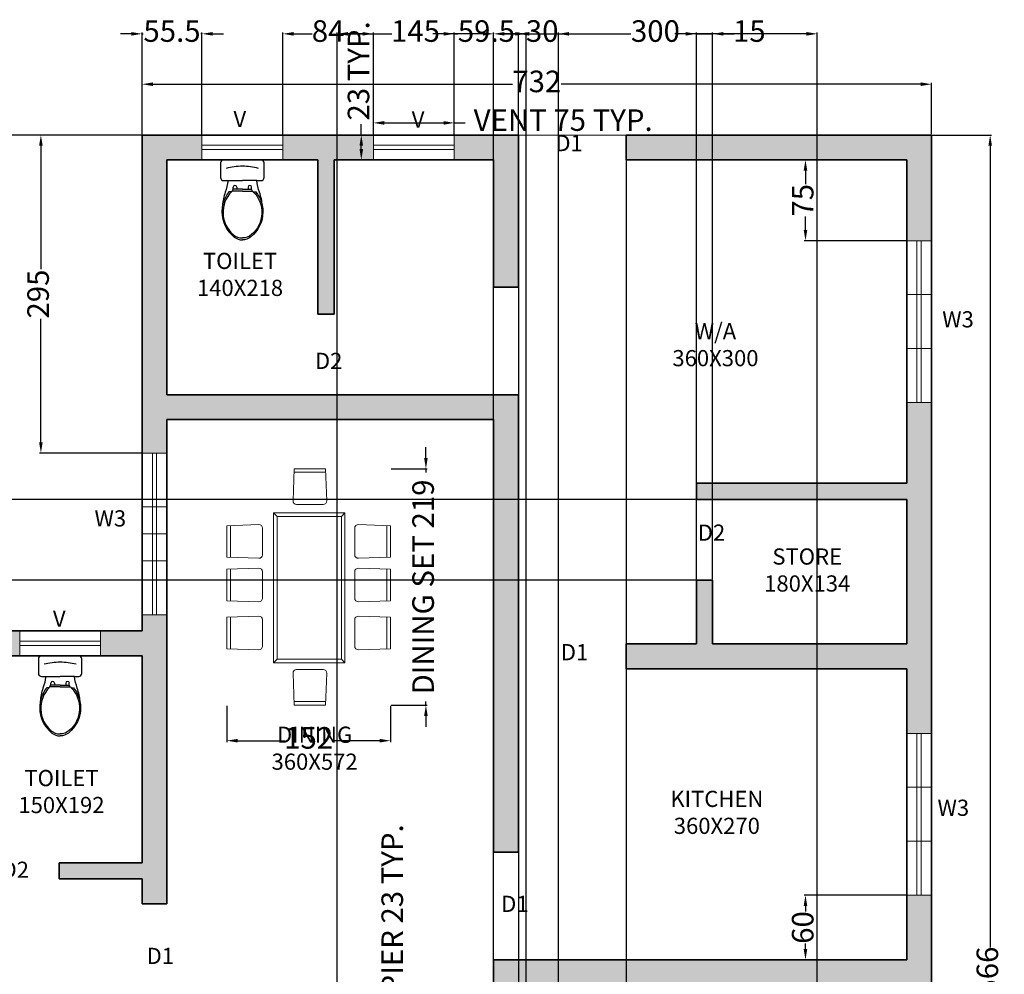
# Model space of a CAD drawing. Units: centimetres. Extents: x 2137 to 3697, y 183 to 2094.
# Tile 8 of 8: x 2745 to 3658, y 1208 to 2094. Entities that reach past the tile are written whole.
import ezdxf

# ---------------------------------------------------------------- set-up
doc = ezdxf.new("R2010")
doc.units = ezdxf.units.CM
for name, color, linetype, lineweight in [('A-ANNO-DIMS', 2, 'Continuous', 18), ('A-ANNO-TEXT', 7, 'Continuous', 18), ('A-AREA-IDEN', 7, 'Continuous', 25), ('A-DOOR', 3, 'Continuous', 18), ('A-FLOR-FIXT', 71, 'Continuous', 18), ('A-FURN', 8, 'Continuous', 18), ('A-GLAZ', 4, 'Continuous', 18), ('A-WALL', 7, 'Continuous', 35), ('A-WALL-PATT', 52, 'Continuous', 13)]:
    doc.layers.add(name, color=color, linetype=linetype, lineweight=lineweight)
doc.layers.add('WC-Detail_dwgmodels.com', color=251, linetype='Continuous')
doc.layers.add('WC-Outline_dwgmodels.com', color=250, linetype='Continuous')
doc.styles.get("Standard").update_dxf_attribs({"font": 'arial.ttf'})
doc.dimstyles.new('ISO-25', dxfattribs={"dimtxt": 20, "dimasz": 10, "dimexe": 1.25, "dimexo": 0.625, "dimtad": 0, "dimtxsty": 'Standard', "dimcen": 2.5, "dimadec": 0, "dimazin": 0, "dimtfac": 1, "dimtmove": 0, "dimatfit": 3, "dimfxl": 1, "dimarcsym": 0})

# ---------------------------------------------------------------- blocks, each defined once
blk = doc.blocks.new('*D1')
at = {"layer": 'A-ANNO-DIMS', "color": 0, "lineweight": -2, "transparency": 16777216}
for p, q in [((2858.02, 1987.3), (2858.02, 2034.96)), ((2868.02, 2033.71), (3201.49, 2033.71)), ((3580.02, 2033.71), (3246.56, 2033.71)), ((3590.02, 1987.3), (3590.02, 2034.96))]:
    blk.add_line(p, q, dxfattribs=at)
at = {"layer": 'A-ANNO-DIMS', "color": 0, "transparency": 16777216}
for points in [[(2868.02, 2035.37), (2868.02, 2032.04), (2858.02, 2033.71)], [(3580.02, 2035.37), (3580.02, 2032.04), (3590.02, 2033.71)]]:
    blk.add_solid(points, dxfattribs=at)
at = {"layer": 'Defpoints', "color": 0, "transparency": 16777216}
for p in [(3590.02, 2033.71), (2858.02, 1986.67), (3590.02, 1986.67)]:
    blk.add_point(p, dxfattribs=at)
at = {"layer": 'A-ANNO-DIMS', "color": 0, "transparency": 16777216, "insert": (3224.02, 2033.71), "char_height": 20, "attachment_point": 5}
blk.add_mtext('732', dxfattribs=at)
blk = doc.blocks.new('*D3')
at = {"layer": 'A-ANNO-DIMS', "color": 0, "lineweight": -2, "transparency": 16777216}
for p, q in [((3590.65, 1986.58), (3645.66, 1986.58)), ((3644.41, 1976.58), (3644.41, 1233.12)), ((3644.41, 430.58), (3644.41, 1174.04)), ((3590.65, 420.58), (3645.66, 420.58))]:
    blk.add_line(p, q, dxfattribs=at)
at = {"layer": 'A-ANNO-DIMS', "color": 0, "transparency": 16777216}
for points in [[(3642.74, 1976.58), (3646.07, 1976.58), (3644.41, 1986.58)], [(3642.74, 430.58), (3646.07, 430.58), (3644.41, 420.58)]]:
    blk.add_solid(points, dxfattribs=at)
at = {"layer": 'Defpoints', "color": 0, "transparency": 16777216}
for p in [(3590.02, 1986.58), (3644.41, 1986.58), (3590.02, 420.58)]:
    blk.add_point(p, dxfattribs=at)
at = {"layer": 'A-ANNO-DIMS', "color": 0, "transparency": 16777216, "insert": (3644.41, 1203.58), "char_height": 20, "attachment_point": 5, "rotation": 90}
blk.add_mtext('1566', dxfattribs=at)
blk = doc.blocks.new('*D6')
at = {"layer": 'A-ANNO-DIMS', "color": 0, "lineweight": -2, "transparency": 16777216}
for p, q in [((2857.4, 1986.58), (2218.37, 1986.58)), ((2219.62, 1976.58), (2219.62, 1779.67)), ((2219.62, 1536.58), (2219.62, 1733.49)), ((2857.4, 1526.58), (2218.37, 1526.58))]:
    blk.add_line(p, q, dxfattribs=at)
at = {"layer": 'A-ANNO-DIMS', "color": 0, "transparency": 16777216}
for points in [[(2217.95, 1976.58), (2221.28, 1976.58), (2219.62, 1986.58)], [(2217.95, 1536.58), (2221.28, 1536.58), (2219.62, 1526.58)]]:
    blk.add_solid(points, dxfattribs=at)
at = {"layer": 'Defpoints', "color": 0, "transparency": 16777216}
for p in [(2858.02, 1986.58), (2219.62, 1526.58), (2858.02, 1526.58)]:
    blk.add_point(p, dxfattribs=at)
at = {"layer": 'A-ANNO-DIMS', "color": 0, "transparency": 16777216, "insert": (2219.62, 1756.58), "char_height": 20, "attachment_point": 5, "rotation": 90}
blk.add_mtext('460', dxfattribs=at)
blk = doc.blocks.new('PAN')
at = {"layer": 'WC-Detail_dwgmodels.com'}
for p, q in [((3002.19, 2116.71), (3003.1, 2118.39)), ((3003.1, 2118.39), (3003.1, 2120.22)), ((3006.38, 2118.39), (3003.1, 2118.39)), ((3006.38, 2120.22), (3006.38, 2118.39)), ((3011.63, 2118.39), (3006.38, 2118.39)), ((3011.63, 2118.39), (3016.89, 2118.39)), ((3016.89, 2120.22), (3016.89, 2118.39)), ((3016.89, 2118.39), (3020.16, 2118.39)), ((3020.16, 2118.39), (3020.16, 2120.22)), ((3021.08, 2116.71), (3020.16, 2118.39))]:
    blk.add_line(p, q, dxfattribs=at)
for points in [[(3001.49, 2116.03, 0.434217), (3003.1, 2076.32, 0.182634), (3011.63, 2073.2, 2.693815)], [(2999.21, 2116.03, 0.094048), (2994, 2106.21, 0.16845)], [(3001.49, 2116.03), (2999.21, 2116.03, 0.416606)], [(3002.19, 2116.71, 0.008985), (3001.49, 2116.03, 0.182634)], [(3011.63, 2116.71), (3002.19, 2116.71, 0.008985)], [(3011.63, 2116.71), (3021.08, 2116.71, -0.444938)], [(3021.78, 2116.03, -0.434217), (3020.16, 2076.32, -0.182634), (3011.63, 2073.2, -2.693815)], [(3021.08, 2116.71, -0.008985), (3021.78, 2116.03, -0.182634)], [(3021.78, 2116.03), (3024.05, 2116.03, -0.416606)], [(3024.05, 2116.03, -0.105447), (3029.64, 2104.91, -0.16845)], [(2994, 2106.21, 0.026594), (2993.22, 2103.13, 0.16845)], [(3029.64, 2104.91, -0.015301), (3030.05, 2103.13, -0.16845)]]:
    blk.add_lwpolyline(points, format="xyb", dxfattribs=at)
for centre, radius, start, end in [((3011.66, 2080.58), 59.08, 90.02796, 104.67123), ((3011.6, 2080.58), 59.08, 75.32877, 89.97204), ((3004.74, 2120.22), 1.64, 0, 180), ((3018.53, 2120.22), 1.64, 0, 180)]:
    blk.add_arc(centre, radius, start, end, dxfattribs=at)
at = {"layer": 'WC-Outline_dwgmodels.com'}
for points in [[(3028.88, 2126.37, 0.414214), (3031.77, 2129.26), (3031.77, 2142.74, 0.414214), (3028.88, 2145.63), (3011.63, 2145.63), (2994.39, 2145.63, 0.414214), (2991.49, 2142.74), (2991.49, 2129.26, 0.414214), (2994.39, 2126.37), (2998.34, 2126.37, -0.052345), (2995.73, 2115.59, 0.071131), (2993.22, 2103.13, 0.160777)], [(2998.34, 2126.37), (3011.63, 2126.37, 0.414214)], [(3024.93, 2126.37), (3011.63, 2126.37, -0.414214)], [(3030.05, 2103.13, 0.071131), (3027.53, 2115.59, -0.052345), (3024.93, 2126.37), (3028.88, 2126.37, 0.414214)], [(2993.22, 2103.13, 0.048023), (2992.66, 2097.45, 0.16845)], [(3030.05, 2103.13, -0.048023), (3030.61, 2097.45, -0.16845)], [(2992.66, 2097.45, 0.230343), (3004.02, 2073.95, 0.16845), (3011.63, 2071.31, 2.883082)], [(3030.61, 2097.45, -0.230343), (3019.25, 2073.95, -0.16845), (3011.63, 2071.31, -2.883082)]]:
    blk.add_lwpolyline(points, format="xyb", dxfattribs=at)
blk = doc.blocks.new('DT')
for p, q in [((2983.25, 1632.88), (2979.94, 1636.19)), ((3042.85, 1632.88), (3046.16, 1636.19)), ((2983.25, 1500.42), (2979.94, 1497.1)), ((3042.85, 1500.42), (3046.16, 1497.1))]:
    blk.add_line(p, q)
for points in [[(3029.23, 1647.36), (3028.24, 1677.05), (2998.99, 1677.05), (2998, 1647.36, 0.424007), (3001.31, 1643.94), (3025.92, 1643.94, 0.424007)], [(2966.34, 1625.25), (2936.65, 1624.26), (2936.65, 1595.01), (2966.34, 1594.02, 0.424007), (2969.77, 1597.33), (2969.77, 1621.94, 0.424007)], [(3058.6, 1625.25), (3088.3, 1624.26), (3088.3, 1595.01), (3058.6, 1594.02, -0.424007), (3055.18, 1597.33), (3055.18, 1621.94, -0.424007)], [(2966.34, 1584.89), (2936.65, 1583.9), (2936.65, 1554.64), (2966.34, 1553.65, 0.424007), (2969.77, 1556.96), (2969.77, 1581.58, 0.424007)], [(3058.6, 1584.89), (3088.3, 1583.9), (3088.3, 1554.64), (3058.6, 1553.65, -0.424007), (3055.18, 1556.96), (3055.18, 1581.58, -0.424007)], [(2966.34, 1540.38), (2936.65, 1539.39), (2936.65, 1510.14), (2966.34, 1509.15, 0.424007), (2969.77, 1512.46), (2969.77, 1537.07, 0.424007)], [(3058.6, 1540.38), (3088.3, 1539.39), (3088.3, 1510.14), (3058.6, 1509.15, -0.424007), (3055.18, 1512.46), (3055.18, 1537.07, -0.424007)], [(3029.23, 1487.43), (3028.24, 1457.73), (2998.99, 1457.73), (2998, 1487.43, -0.424007), (3001.31, 1490.85), (3025.92, 1490.85, -0.424007)]]:
    blk.add_lwpolyline(points, format="xyb", close=True)
for points in [[(2998.88, 1673.74), (3028.35, 1673.74)], [(2939.96, 1594.9), (2939.96, 1624.37)], [(3084.99, 1594.9), (3084.99, 1624.37)], [(2939.96, 1554.53), (2939.96, 1584.01)], [(3084.99, 1554.53), (3084.99, 1584.01)], [(2939.96, 1510.03), (2939.96, 1539.5)], [(3084.99, 1510.03), (3084.99, 1539.5)], [(2998.88, 1461.04), (3028.35, 1461.04)]]:
    blk.add_lwpolyline(points)
for points in [[(2979.94, 1497.1), (3046.16, 1497.1), (3046.16, 1636.19), (2979.94, 1636.19)], [(2983.25, 1500.42), (3042.85, 1500.42), (3042.85, 1632.88), (2983.25, 1632.88)]]:
    blk.add_lwpolyline(points, close=True)
blk = doc.blocks.new('WIN-W3-150CM')
for p, q in [((0, 23), (0, 0)), ((50, 23), (50, 0)), ((100, 23), (100, 0)), ((150, 23), (150, 0)), ((0, 13.5), (150, 13.5)), ((0, 9.5), (150, 9.5))]:
    blk.add_line(p, q)
blk = doc.blocks.new('VENT-75CM')
for p, q in [((0, 0), (0, 23)), ((75, 0), (75, 23)), ((0, 13.5), (75, 13.5)), ((0, 9.5), (75, 9.5))]:
    blk.add_line(p, q)
blk = doc.blocks.new('*D22')
at = {"layer": 'A-ANNO-DIMS', "color": 0, "lineweight": -2, "transparency": 16777216}
for p, q in [((3072.52, 1987.2), (3072.52, 1999.08)), ((3082.52, 1997.83), (3137.52, 1997.83)), ((3147.52, 1987.2), (3147.52, 1999.08)), ((3147.52, 1997.83), (3157.52, 1997.83))]:
    blk.add_line(p, q, dxfattribs=at)
at = {"layer": 'A-ANNO-DIMS', "color": 0, "transparency": 16777216}
for points in [[(3082.52, 1999.5), (3082.52, 1996.16), (3072.52, 1997.83)], [(3137.52, 1999.5), (3137.52, 1996.16), (3147.52, 1997.83)]]:
    blk.add_solid(points, dxfattribs=at)
at = {"layer": 'Defpoints', "color": 0, "transparency": 16777216}
for p in [(3147.52, 1997.83), (3072.52, 1986.58), (3147.52, 1986.58)]:
    blk.add_point(p, dxfattribs=at)
at = {"layer": 'A-ANNO-DIMS', "color": 0, "transparency": 16777216, "insert": (3248.48, 1997.83), "char_height": 20, "attachment_point": 5}
blk.add_mtext('VENT 75 TYP.', dxfattribs=at)
blk = doc.blocks.new('*D23')
at = {"layer": 'A-ANNO-DIMS', "color": 0, "lineweight": -2, "transparency": 16777216}
for p, q in [((3061.27, 1986.58), (3061.27, 1996.58)), ((3071.9, 1986.58), (3060.02, 1986.58)), ((3061.27, 1973.58), (3061.27, 1976.58)), ((3071.9, 1963.58), (3060.02, 1963.58))]:
    blk.add_line(p, q, dxfattribs=at)
at = {"layer": 'A-ANNO-DIMS', "color": 0, "transparency": 16777216}
for points in [[(3059.61, 1976.58), (3062.94, 1976.58), (3061.27, 1986.58)], [(3059.61, 1973.58), (3062.94, 1973.58), (3061.27, 1963.58)]]:
    blk.add_solid(points, dxfattribs=at)
at = {"layer": 'Defpoints', "color": 0, "transparency": 16777216}
for p in [(3061.27, 1986.58), (3072.52, 1986.58), (3072.52, 1963.58)]:
    blk.add_point(p, dxfattribs=at)
at = {"layer": 'A-ANNO-DIMS', "color": 0, "transparency": 16777216, "insert": (3061.27, 2046.05), "char_height": 20, "attachment_point": 5, "rotation": 90}
blk.add_mtext('23 TYP.', dxfattribs=at)
blk = doc.blocks.new('*D28')
at = {"layer": 'A-ANNO-DIMS', "color": 0, "lineweight": -2, "transparency": 16777216}
for p, q in [((3092.57, 1173.58), (3092.57, 1183.58)), ((3089.74, 1173.58), (3093.82, 1173.58)), ((3092.57, 1160.58), (3092.57, 1163.58)), ((3089.74, 1150.58), (3093.82, 1150.58))]:
    blk.add_line(p, q, dxfattribs=at)
at = {"layer": 'A-ANNO-DIMS', "color": 0, "transparency": 16777216}
for points in [[(3090.9, 1163.58), (3094.23, 1163.58), (3092.57, 1173.58)], [(3090.9, 1160.58), (3094.23, 1160.58), (3092.57, 1150.58)]]:
    blk.add_solid(points, dxfattribs=at)
at = {"layer": 'Defpoints', "color": 0, "transparency": 16777216}
for p in [(3089.12, 1173.58), (3092.57, 1173.58), (3089.12, 1150.58)]:
    blk.add_point(p, dxfattribs=at)
at = {"layer": 'A-ANNO-DIMS', "color": 0, "transparency": 16777216, "insert": (3092.57, 1268.87), "char_height": 20, "attachment_point": 5, "rotation": 90}
blk.add_mtext('PIER 23 TYP.', dxfattribs=at)
blk = doc.blocks.new('*D36')
at = {"layer": 'A-ANNO-DIMS', "color": 0, "lineweight": -2, "transparency": 16777216}
for p, q in [((3121.19, 1687.05), (3121.19, 1697.05)), ((3088.92, 1677.05), (3122.44, 1677.05)), ((3121.19, 1677.05), (3121.19, 1673.46)), ((3121.19, 1457.73), (3121.19, 1461.32)), ((3088.92, 1457.73), (3122.44, 1457.73)), ((3121.19, 1447.73), (3121.19, 1437.73))]:
    blk.add_line(p, q, dxfattribs=at)
at = {"layer": 'A-ANNO-DIMS', "color": 0, "transparency": 16777216}
for points in [[(3119.53, 1687.05), (3122.86, 1687.05), (3121.19, 1677.05)], [(3119.53, 1447.73), (3122.86, 1447.73), (3121.19, 1457.73)]]:
    blk.add_solid(points, dxfattribs=at)
at = {"layer": 'Defpoints', "color": 0, "transparency": 16777216}
for p in [(3088.3, 1677.05), (3121.19, 1677.05), (3088.3, 1457.73)]:
    blk.add_point(p, dxfattribs=at)
at = {"layer": 'A-ANNO-DIMS', "color": 0, "transparency": 16777216, "insert": (3121.19, 1567.39), "char_height": 20, "attachment_point": 5, "rotation": 90}
blk.add_mtext('DINING SET 219', dxfattribs=at)
blk = doc.blocks.new('*D37')
at = {"layer": 'A-ANNO-DIMS', "color": 0, "lineweight": -2, "transparency": 16777216}
for p, q in [((2936.65, 1457.11), (2936.65, 1423.59)), ((3088.3, 1457.11), (3088.3, 1423.59)), ((2946.65, 1424.84), (2990.8, 1424.84)), ((3078.3, 1424.84), (3034.15, 1424.84))]:
    blk.add_line(p, q, dxfattribs=at)
at = {"layer": 'A-ANNO-DIMS', "color": 0, "transparency": 16777216}
for points in [[(2946.65, 1426.5), (2946.65, 1423.17), (2936.65, 1424.84)], [(3078.3, 1426.5), (3078.3, 1423.17), (3088.3, 1424.84)]]:
    blk.add_solid(points, dxfattribs=at)
at = {"layer": 'Defpoints', "color": 0, "transparency": 16777216}
for p in [(2936.65, 1457.73), (3088.3, 1457.73), (3088.3, 1424.84)]:
    blk.add_point(p, dxfattribs=at)
at = {"layer": 'A-ANNO-DIMS', "color": 0, "transparency": 16777216, "insert": (3012.47, 1424.84), "char_height": 20, "attachment_point": 5}
blk.add_mtext('152', dxfattribs=at)
blk = doc.blocks.new('*D38')
at = {"layer": 'A-ANNO-DIMS', "color": 0, "lineweight": -2, "transparency": 16777216}
for p, q in [((2857.4, 1986.58), (2174.92, 1986.58)), ((2176.17, 1976.58), (2176.17, 1171.09)), ((2176.17, 306.58), (2176.17, 1112.07)), ((2269.4, 296.58), (2174.92, 296.58))]:
    blk.add_line(p, q, dxfattribs=at)
at = {"layer": 'A-ANNO-DIMS', "color": 0, "transparency": 16777216}
for points in [[(2174.51, 1976.58), (2177.84, 1976.58), (2176.17, 1986.58)], [(2174.51, 306.58), (2177.84, 306.58), (2176.17, 296.58)]]:
    blk.add_solid(points, dxfattribs=at)
at = {"layer": 'Defpoints', "color": 0, "transparency": 16777216}
for p in [(2176.17, 1986.58), (2858.02, 1986.58), (2270.02, 296.58)]:
    blk.add_point(p, dxfattribs=at)
at = {"layer": 'A-ANNO-DIMS', "color": 0, "transparency": 16777216, "insert": (2176.17, 1141.58), "char_height": 20, "attachment_point": 5, "rotation": 90}
blk.add_mtext('1690', dxfattribs=at)
blk = doc.blocks.new('*D39')
at = {"layer": 'A-ANNO-DIMS', "color": 0, "lineweight": -2, "transparency": 16777216}
for p, q in [((3039.02, 600.2), (3039.02, 2081.68)), ((3184.02, 600.2), (3184.02, 2081.68)), ((3049.02, 2080.43), (3089.67, 2080.43)), ((3174.02, 2080.43), (3133.38, 2080.43))]:
    blk.add_line(p, q, dxfattribs=at)
at = {"layer": 'A-ANNO-DIMS', "color": 0, "transparency": 16777216}
for points in [[(3049.02, 2082.1), (3049.02, 2078.76), (3039.02, 2080.43)], [(3174.02, 2082.1), (3174.02, 2078.76), (3184.02, 2080.43)]]:
    blk.add_solid(points, dxfattribs=at)
at = {"layer": 'Defpoints', "color": 0, "transparency": 16777216}
for p in [(3184.02, 2080.43), (3039.02, 599.58), (3184.02, 599.58)]:
    blk.add_point(p, dxfattribs=at)
at = {"layer": 'A-ANNO-DIMS', "color": 0, "transparency": 16777216, "insert": (3111.52, 2080.43), "char_height": 20, "attachment_point": 5}
blk.add_mtext('145', dxfattribs=at)
blk = doc.blocks.new('*D40')
at = {"layer": 'A-ANNO-DIMS', "color": 0, "lineweight": -2, "transparency": 16777216}
for p, q in [((3207.02, 1985.95), (3207.02, 201.48)), ((3307.02, 1985.95), (3307.02, 201.48)), ((3217.02, 202.73), (3235.28, 202.73)), ((3297.02, 202.73), (3278.77, 202.73))]:
    blk.add_line(p, q, dxfattribs=at)
at = {"layer": 'A-ANNO-DIMS', "color": 0, "transparency": 16777216}
for points in [[(3217.02, 204.4), (3217.02, 201.06), (3207.02, 202.73)], [(3297.02, 204.4), (3297.02, 201.06), (3307.02, 202.73)]]:
    blk.add_solid(points, dxfattribs=at)
at = {"layer": 'Defpoints', "color": 0, "transparency": 16777216}
for p in [(3207.02, 1986.58), (3307.02, 1986.58), (3307.02, 202.73)]:
    blk.add_point(p, dxfattribs=at)
at = {"layer": 'A-ANNO-DIMS', "color": 0, "transparency": 16777216, "insert": (3257.02, 202.73), "char_height": 20, "attachment_point": 5}
blk.add_mtext('100', dxfattribs=at)
blk = doc.blocks.new('*D41')
at = {"layer": 'A-ANNO-DIMS', "color": 0, "lineweight": -2, "transparency": 16777216}
for p, q in [((3371.4, 1648.58), (2174.92, 1648.58)), ((2176.17, 1638.58), (2176.17, 1626.02)), ((2176.17, 1583.58), (2176.17, 1596.14)), ((3371.4, 1573.58), (2174.92, 1573.58))]:
    blk.add_line(p, q, dxfattribs=at)
at = {"layer": 'A-ANNO-DIMS', "color": 0, "transparency": 16777216}
for points in [[(2174.51, 1638.58), (2177.84, 1638.58), (2176.17, 1648.58)], [(2174.51, 1583.58), (2177.84, 1583.58), (2176.17, 1573.58)]]:
    blk.add_solid(points, dxfattribs=at)
at = {"layer": 'Defpoints', "color": 0, "transparency": 16777216}
for p in [(2176.17, 1648.58), (3372.02, 1648.58), (3372.02, 1573.58)]:
    blk.add_point(p, dxfattribs=at)
at = {"layer": 'A-ANNO-DIMS', "color": 0, "transparency": 16777216, "insert": (2176.17, 1611.08), "char_height": 20, "attachment_point": 5, "rotation": 90}
blk.add_mtext('75', dxfattribs=at)
blk = doc.blocks.new('*D43')
at = {"layer": 'A-ANNO-DIMS', "color": 0, "lineweight": -2, "transparency": 16777216}
for p, q in [((3184.02, 800.2), (3184.02, 2081.68)), ((3484.02, 800.2), (3484.02, 2081.68)), ((3194.02, 2080.43), (3311.34, 2080.43)), ((3474.02, 2080.43), (3356.7, 2080.43))]:
    blk.add_line(p, q, dxfattribs=at)
at = {"layer": 'A-ANNO-DIMS', "color": 0, "transparency": 16777216}
for points in [[(3194.02, 2082.1), (3194.02, 2078.76), (3184.02, 2080.43)], [(3474.02, 2082.1), (3474.02, 2078.76), (3484.02, 2080.43)]]:
    blk.add_solid(points, dxfattribs=at)
at = {"layer": 'Defpoints', "color": 0, "transparency": 16777216}
for p in [(3484.02, 2080.43), (3184.02, 799.58), (3484.02, 799.58)]:
    blk.add_point(p, dxfattribs=at)
at = {"layer": 'A-ANNO-DIMS', "color": 0, "transparency": 16777216, "insert": (3334.02, 2080.43), "char_height": 20, "attachment_point": 5}
blk.add_mtext('300', dxfattribs=at)
blk = doc.blocks.new('*D44')
at = {"layer": 'A-ANNO-DIMS', "color": 0, "lineweight": -2, "transparency": 16777216}
for p, q in [((3214.02, 800.2), (3214.02, 2081.68)), ((3244.02, 800.2), (3244.02, 2081.68)), ((3204.02, 2080.43), (3194.02, 2080.43)), ((3214.02, 2080.43), (3214.11, 2080.43)), ((3244.02, 2080.43), (3243.93, 2080.43)), ((3254.02, 2080.43), (3264.02, 2080.43))]:
    blk.add_line(p, q, dxfattribs=at)
at = {"layer": 'A-ANNO-DIMS', "color": 0, "transparency": 16777216}
for points in [[(3204.02, 2082.1), (3204.02, 2078.76), (3214.02, 2080.43)], [(3254.02, 2082.1), (3254.02, 2078.76), (3244.02, 2080.43)]]:
    blk.add_solid(points, dxfattribs=at)
at = {"layer": 'Defpoints', "color": 0, "transparency": 16777216}
for p in [(3244.02, 2080.43), (3214.02, 799.58), (3244.02, 799.58)]:
    blk.add_point(p, dxfattribs=at)
at = {"layer": 'A-ANNO-DIMS', "color": 0, "transparency": 16777216, "insert": (3229.02, 2080.43), "char_height": 20, "attachment_point": 5}
blk.add_mtext('30', dxfattribs=at)
blk = doc.blocks.new('*D47')
at = {"layer": 'A-ANNO-DIMS', "color": 0, "lineweight": -2, "transparency": 16777216}
for p, q in [((3566.4, 1281.58), (3471.92, 1281.58)), ((3473.17, 1271.58), (3473.17, 1266.55)), ((3473.17, 1231.58), (3473.17, 1236.61)), ((3566.4, 1221.58), (3471.92, 1221.58))]:
    blk.add_line(p, q, dxfattribs=at)
at = {"layer": 'A-ANNO-DIMS', "color": 0, "transparency": 16777216}
for points in [[(3471.51, 1271.58), (3474.84, 1271.58), (3473.17, 1281.58)], [(3471.51, 1231.58), (3474.84, 1231.58), (3473.17, 1221.58)]]:
    blk.add_solid(points, dxfattribs=at)
at = {"layer": 'Defpoints', "color": 0, "transparency": 16777216}
for p in [(3473.17, 1281.58), (3567.02, 1281.58), (3567.02, 1221.58)]:
    blk.add_point(p, dxfattribs=at)
at = {"layer": 'A-ANNO-DIMS', "color": 0, "transparency": 16777216, "insert": (3473.17, 1251.58), "char_height": 20, "attachment_point": 5, "rotation": 90}
blk.add_mtext('60', dxfattribs=at)
blk = doc.blocks.new('*D48')
at = {"layer": 'A-ANNO-DIMS', "color": 0, "lineweight": -2, "transparency": 16777216}
for p, q in [((3566.4, 1963.58), (3471.92, 1963.58)), ((3473.17, 1953.58), (3473.17, 1941.02)), ((3473.17, 1898.58), (3473.17, 1911.14)), ((3566.4, 1888.58), (3471.92, 1888.58))]:
    blk.add_line(p, q, dxfattribs=at)
at = {"layer": 'A-ANNO-DIMS', "color": 0, "transparency": 16777216}
for points in [[(3471.51, 1953.58), (3474.84, 1953.58), (3473.17, 1963.58)], [(3471.51, 1898.58), (3474.84, 1898.58), (3473.17, 1888.58)]]:
    blk.add_solid(points, dxfattribs=at)
at = {"layer": 'Defpoints', "color": 0, "transparency": 16777216}
for p in [(3473.17, 1963.58), (3567.02, 1963.58), (3567.02, 1888.58)]:
    blk.add_point(p, dxfattribs=at)
at = {"layer": 'A-ANNO-DIMS', "color": 0, "transparency": 16777216, "insert": (3473.17, 1926.08), "char_height": 20, "attachment_point": 5, "rotation": 90}
blk.add_mtext('75', dxfattribs=at)
blk = doc.blocks.new('*D57')
at = {"layer": 'A-ANNO-DIMS', "color": 0, "lineweight": -2, "transparency": 16777216}
for p, q in [((2857.4, 1986.58), (2762.92, 1986.58)), ((2764.17, 1976.58), (2764.17, 1862.06)), ((2764.17, 1701.6), (2764.17, 1816.13)), ((2857.4, 1691.6), (2762.92, 1691.6))]:
    blk.add_line(p, q, dxfattribs=at)
at = {"layer": 'A-ANNO-DIMS', "color": 0, "transparency": 16777216}
for points in [[(2762.51, 1976.58), (2765.84, 1976.58), (2764.17, 1986.58)], [(2762.51, 1701.6), (2765.84, 1701.6), (2764.17, 1691.6)]]:
    blk.add_solid(points, dxfattribs=at)
at = {"layer": 'Defpoints', "color": 0, "transparency": 16777216}
for p in [(2764.17, 1986.58), (2858.02, 1986.58), (2858.02, 1691.6)]:
    blk.add_point(p, dxfattribs=at)
at = {"layer": 'A-ANNO-DIMS', "color": 0, "transparency": 16777216, "insert": (2764.17, 1839.09), "char_height": 20, "attachment_point": 5, "rotation": 90}
blk.add_mtext('295', dxfattribs=at)
blk = doc.blocks.new('*D58')
at = {"layer": 'A-ANNO-DIMS', "color": 0, "lineweight": -2, "transparency": 16777216}
for p, q in [((2858.02, 1987.2), (2858.02, 2081.68)), ((2913.52, 1987.2), (2913.52, 2081.68)), ((2848.02, 2080.43), (2838.02, 2080.43)), ((2858.02, 2080.43), (2859.1, 2080.43)), ((2913.52, 2080.43), (2912.45, 2080.43)), ((2923.52, 2080.43), (2933.52, 2080.43))]:
    blk.add_line(p, q, dxfattribs=at)
at = {"layer": 'A-ANNO-DIMS', "color": 0, "transparency": 16777216}
for points in [[(2848.02, 2082.1), (2848.02, 2078.76), (2858.02, 2080.43)], [(2923.52, 2082.1), (2923.52, 2078.76), (2913.52, 2080.43)]]:
    blk.add_solid(points, dxfattribs=at)
at = {"layer": 'Defpoints', "color": 0, "transparency": 16777216}
for p in [(2913.52, 2080.43), (2858.02, 1986.58), (2913.52, 1986.58)]:
    blk.add_point(p, dxfattribs=at)
at = {"layer": 'A-ANNO-DIMS', "color": 0, "transparency": 16777216, "insert": (2885.77, 2080.43), "char_height": 20, "attachment_point": 5}
blk.add_mtext('55.5', dxfattribs=at)
blk = doc.blocks.new('*D59')
at = {"layer": 'A-ANNO-DIMS', "color": 0, "lineweight": -2, "transparency": 16777216}
for p, q in [((2988.52, 1987.2), (2988.52, 2081.68)), ((3072.52, 1987.2), (3072.52, 2081.68)), ((2998.52, 2080.43), (3015.6, 2080.43)), ((3062.52, 2080.43), (3045.44, 2080.43))]:
    blk.add_line(p, q, dxfattribs=at)
at = {"layer": 'A-ANNO-DIMS', "color": 0, "transparency": 16777216}
for points in [[(2998.52, 2082.1), (2998.52, 2078.76), (2988.52, 2080.43)], [(3062.52, 2082.1), (3062.52, 2078.76), (3072.52, 2080.43)]]:
    blk.add_solid(points, dxfattribs=at)
at = {"layer": 'Defpoints', "color": 0, "transparency": 16777216}
for p in [(3072.52, 2080.43), (2988.52, 1986.58), (3072.52, 1986.58)]:
    blk.add_point(p, dxfattribs=at)
at = {"layer": 'A-ANNO-DIMS', "color": 0, "transparency": 16777216, "insert": (3030.52, 2080.43), "char_height": 20, "attachment_point": 5}
blk.add_mtext('84', dxfattribs=at)
blk = doc.blocks.new('*D60')
at = {"layer": 'A-ANNO-DIMS', "color": 0, "lineweight": -2, "transparency": 16777216}
for p, q in [((3147.52, 1987.2), (3147.52, 2081.68)), ((3207.02, 1987.2), (3207.02, 2081.68)), ((3137.52, 2080.43), (3127.52, 2080.43)), ((3147.52, 2080.43), (3150.6, 2080.43)), ((3207.02, 2080.43), (3203.95, 2080.43)), ((3217.02, 2080.43), (3227.02, 2080.43))]:
    blk.add_line(p, q, dxfattribs=at)
at = {"layer": 'A-ANNO-DIMS', "color": 0, "transparency": 16777216}
for points in [[(3137.52, 2082.1), (3137.52, 2078.76), (3147.52, 2080.43)], [(3217.02, 2082.1), (3217.02, 2078.76), (3207.02, 2080.43)]]:
    blk.add_solid(points, dxfattribs=at)
at = {"layer": 'Defpoints', "color": 0, "transparency": 16777216}
for p in [(3207.02, 2080.43), (3147.52, 1986.58), (3207.02, 1986.58)]:
    blk.add_point(p, dxfattribs=at)
at = {"layer": 'A-ANNO-DIMS', "color": 0, "transparency": 16777216, "insert": (3177.27, 2080.43), "char_height": 20, "attachment_point": 5}
blk.add_mtext('59.5', dxfattribs=at)
blk = doc.blocks.new('*D61')
at = {"layer": 'A-ANNO-DIMS', "color": 0, "lineweight": -2, "transparency": 16777216}
for p, q in [((3372.02, 1574.2), (3372.02, 2081.68)), ((3387.02, 1574.2), (3387.02, 2081.68)), ((3362.02, 2080.43), (3352.02, 2080.43)), ((3372.02, 2080.43), (3387.02, 2080.43)), ((3397.02, 2080.43), (3407.02, 2080.43))]:
    blk.add_line(p, q, dxfattribs=at)
at = {"layer": 'A-ANNO-DIMS', "color": 0, "transparency": 16777216}
for points in [[(3362.02, 2082.1), (3362.02, 2078.76), (3372.02, 2080.43)], [(3397.02, 2082.1), (3397.02, 2078.76), (3387.02, 2080.43)]]:
    blk.add_solid(points, dxfattribs=at)
at = {"layer": 'Defpoints', "color": 0, "transparency": 16777216}
for p in [(3387.02, 2080.43), (3372.02, 1573.58), (3387.02, 1573.58)]:
    blk.add_point(p, dxfattribs=at)
at = {"layer": 'A-ANNO-DIMS', "color": 0, "transparency": 16777216, "insert": (3421.11, 2080.43), "char_height": 20, "attachment_point": 5}
blk.add_mtext('15', dxfattribs=at)

msp = doc.modelspace()

# ---------------------------------------------------------------- hatches: boundary and pattern name
at = {"layer": 'A-WALL-PATT'}
h = msp.add_hatch(color=256, dxfattribs=at)
h.dxf.hatch_style = 1
h.paths.add_polyline_path([(2413.023, 1526.579), (2270.023, 1526.579), (2270.023, 1413.579), (2293.023, 1413.579), (2293.023, 1503.579), (2413.023, 1503.579)])
h.paths.add_polyline_path([(2744.523, 1526.579), (2563.023, 1526.579), (2563.023, 1503.579), (2638.023, 1503.579), (2683.023, 1503.579), (2683.023, 1296.579), (2706.023, 1296.579), (2706.023, 1503.579), (2744.523, 1503.579)])
h.paths.add_polyline_path([(2881.023, 1541.602), (2858.023, 1541.602), (2858.023, 1526.579), (2819.523, 1526.579), (2819.523, 1503.579), (2858.023, 1503.579), (2858.023, 1311.579), (2781.023, 1311.579), (2781.023, 1296.579), (2858.023, 1296.579), (2858.023, 1273.579), (2881.023, 1273.579)])
h.paths.add_polyline_path([(3207.023, 1745.579), (2881.023, 1745.579), (2881.023, 1963.579), (2913.523, 1963.579), (2913.523, 1986.579), (2858.023, 1986.579), (2858.023, 1691.602), (2881.023, 1691.602), (2881.023, 1722.579), (3184.023, 1722.579), (3184.023, 1321.579), (3207.023, 1321.579)])
h.paths.add_polyline_path([(3072.523, 1986.579), (2988.523, 1986.579), (2988.523, 1963.579), (3021.023, 1963.579), (3021.023, 1820.579), (3036.023, 1820.579), (3036.023, 1963.579), (3072.523, 1963.579)], flags=17)
h.paths.add_polyline_path([(3207.023, 1986.579), (3147.523, 1986.579), (3147.523, 1963.579), (3184.023, 1963.579), (3184.023, 1845.579), (3207.023, 1845.579)], flags=17)
h.paths.add_polyline_path([(3590.023, 1986.579), (3307.023, 1986.579), (3307.023, 1963.579), (3567.023, 1963.579), (3567.023, 1888.579), (3590.023, 1888.579), (3590.023, 1963.579)])
h.paths.add_polyline_path([(3590.023, 1738.579), (3567.023, 1738.579), (3567.023, 1663.579), (3372.023, 1663.579), (3372.023, 1648.579), (3567.023, 1648.579), (3567.023, 1514.579), (3387.023, 1514.579), (3387.023, 1573.579), (3372.023, 1573.579), (3372.023, 1514.579), (3307.023, 1514.579), (3307.023, 1491.579), (3567.023, 1491.579), (3567.023, 1431.579), (3590.023, 1431.579)])
h.paths.add_polyline_path([(3590.023, 1281.579), (3567.023, 1281.579), (3567.023, 1221.579), (3184.023, 1221.579), (3184.023, 922.579), (3207.023, 922.579), (3207.023, 1198.579), (3567.023, 1198.579), (3567.023, 1055.075), (3590.023, 1055.075)])
h.paths.add_polyline_path([(3590.023, 905.075), (3567.023, 905.075), (3567.023, 774.852), (3590.023, 774.852)])
h.paths.add_polyline_path([(3590.023, 624.852), (3567.023, 624.852), (3567.023, 599.579), (3184.023, 599.579), (3184.023, 576.579), (3590.023, 576.579)])
h.paths.add_polyline_path([(3590.023, 443.579), (3567.023, 443.579), (3567.023, 420.579), (3590.023, 420.579)])
h.paths.add_polyline_path([(3225.908, 443.579), (3202.908, 443.579), (3202.908, 420.579), (3225.908, 420.579)])
h.paths.add_polyline_path([(3039.023, 599.579), (3016.023, 599.579), (3016.023, 443.579), (2937.023, 443.579), (2937.023, 420.579), (3039.023, 420.579)])
h.paths.add_polyline_path([(2787.023, 443.579), (2708.023, 443.579), (2708.023, 850.579), (2685.023, 850.579), (2685.023, 319.579), (2564.023, 319.579), (2564.023, 296.579), (2708.023, 296.579), (2708.023, 420.579), (2787.023, 420.579)])
h.paths.add_polyline_path([(2414.023, 319.579), (2293.023, 319.579), (2293.023, 412.079), (2270.023, 412.079), (2270.023, 296.579), (2414.023, 296.579)])
h.paths.add_polyline_path([(2592.023, 677.579), (2293.023, 677.579), (2293.023, 715.079), (2270.023, 715.079), (2270.023, 562.079), (2293.023, 562.079), (2293.023, 637.079), (2293.023, 654.579), (2592.023, 654.579)])
h.paths.add_polyline_path([(2592.023, 850.579), (2526.773, 850.579), (2526.441, 850.508), (2377.032, 850.508), (2293.023, 850.579), (2293.023, 925.579), (2270.023, 925.579), (2270.023, 790.079), (2293.023, 790.079), (2293.023, 827.579), (2569.023, 827.579), (2569.023, 752.579), (2592.023, 752.579)])
h.paths.add_polyline_path([(2293.023, 1263.579), (2270.023, 1263.579), (2270.023, 1075.579), (2293.023, 1075.579), (2293.023, 1150.579), (2881.023, 1150.579), (2881.023, 1173.579), (2293.023, 1173.579)])

# ---------------------------------------------------------------- linework, layer by layer
at = {"layer": 'A-DOOR'}
msp.add_line((3207.023, 1986.579), (3307.023, 1986.579), dxfattribs=at)
at = {"layer": 'A-GLAZ'}
for p, q in [((2858.023, 1691.602), (2881.023, 1691.602)), ((2867.523, 1541.602), (2867.523, 1691.602)), ((2871.523, 1541.602), (2871.523, 1691.602)), ((2858.023, 1641.602), (2881.023, 1641.602)), ((2881.023, 1616.602), (2858.023, 1616.602)), ((2858.023, 1591.602), (2881.023, 1591.602)), ((2858.023, 1541.602), (2881.023, 1541.602))]:
    msp.add_line(p, q, dxfattribs=at)
at = {"layer": 'A-WALL'}
for p, q in [((2858.023, 1986.579), (3207.023, 1986.579)), ((2858.023, 1986.579), (2858.023, 1526.579)), ((3207.023, 1986.579), (3207.023, 1845.579)), ((3307.023, 1986.579), (3307.023, 1963.579)), ((3307.023, 1986.579), (3590.023, 1986.579)), ((3590.023, 1986.579), (3590.023, 420.579)), ((2881.023, 1963.579), (2881.023, 1745.579)), ((2881.023, 1963.579), (3021.023, 1963.579)), ((3021.023, 1963.579), (3021.023, 1820.579)), ((3036.023, 1963.579), (3036.023, 1820.579)), ((3036.023, 1963.579), (3184.023, 1963.579)), ((3184.023, 1963.579), (3184.023, 1845.579)), ((3307.023, 1963.579), (3567.023, 1963.579)), ((3567.023, 1963.579), (3567.023, 1663.579)), ((3590.023, 1963.579), (3590.023, 420.579)), ((3184.023, 1845.579), (3207.023, 1845.579)), ((3021.023, 1820.579), (3036.023, 1820.579)), ((2881.023, 1745.579), (3207.023, 1745.579)), ((3207.023, 1745.579), (3207.023, 1321.579)), ((2881.023, 1722.579), (3184.023, 1722.579)), ((2881.023, 1722.579), (2881.023, 1273.579)), ((3184.023, 1722.579), (3184.023, 1321.579)), ((3372.023, 1663.579), (3567.023, 1663.579)), ((3372.023, 1663.579), (3372.023, 1648.579)), ((3372.023, 1648.579), (3567.023, 1648.579)), ((3567.023, 1648.579), (3567.023, 1514.579)), ((3372.023, 1573.579), (3387.023, 1573.579)), ((3372.023, 1573.579), (3372.023, 1514.579)), ((3387.023, 1573.579), (3387.023, 1514.579)), ((2270.023, 1526.579), (2858.023, 1526.579)), ((3307.023, 1514.579), (3307.023, 1491.579)), ((3307.023, 1514.579), (3372.023, 1514.579)), ((3387.023, 1514.579), (3567.023, 1514.579)), ((2706.023, 1503.579), (2858.023, 1503.579)), ((2858.023, 1503.579), (2858.023, 1311.579)), ((3307.023, 1491.579), (3567.023, 1491.579)), ((3567.023, 1491.579), (3567.023, 1221.579)), ((3184.023, 1321.579), (3207.023, 1321.579)), ((2781.023, 1311.579), (2781.023, 1296.579)), ((2781.023, 1311.579), (2858.023, 1311.579)), ((2781.023, 1296.579), (2858.023, 1296.579)), ((2858.023, 1296.579), (2858.023, 1273.579)), ((2858.023, 1273.579), (2881.023, 1273.579)), ((3184.023, 1221.579), (3567.023, 1221.579)), ((3184.023, 1221.579), (3184.023, 922.579))]:
    msp.add_line(p, q, dxfattribs=at)

# ---------------------------------------------------------------- block references
at = {"layer": 'A-FLOR-FIXT'}
for p in [(-60.611, -182.049), (-229.611, -642.049)]:
    msp.add_blockref('PAN', p, dxfattribs=at)
at = {"layer": 'A-FURN'}
msp.add_blockref('DT', (0, 0), dxfattribs=at)
at = {"layer": 'A-GLAZ'}
for p in [(2913.523, 1963.579), (3072.523, 1963.579), (2744.523, 1503.579)]:
    msp.add_blockref('VENT-75CM', p, dxfattribs=at)
for p, rotation in [((3590.023, 1738.579), 89.9999999999996), ((3590.023, 1281.579), 89.99999999999996)]:
    msp.add_blockref('WIN-W3-150CM', p, dxfattribs=dict(at, rotation=rotation))

# ---------------------------------------------------------------- texts
at = {"layer": 'A-ANNO-TEXT', "char_height": 15, "attachment_point": 1}
for s, insert in [('\\pxqc;V', (2924.144, 2008.901)), ('\\pxqc;V', (3089.449, 2008.454)), ('\\pxqc;D1', (3229.487, 1986.579)), ('\\pxqc;W3', (3590.142, 1823.145)), ('\\pxqc;D2', (3006.566, 1784.603)), ('\\pxqc;W3', (2804.083, 1638.499)), ('\\pxqc;D2', (3361.538, 1625.302)), ('\\pxqc;V', (2756.722, 1545.52)), ('\\pxqc;D1', (3234.554, 1514.443)), ('\\pxqc;W3', (3585.787, 1370.122)), ('\\pxqc;D2', (2715.927, 1312.635)), ('\\pxqc;D1', (3179.228, 1281.007)), ('\\pxqc;D1', (2850.461, 1232.722))]:
    msp.add_mtext_dynamic_manual_height_columns(s, width=48.94887, gutter_width=12.5, heights=[0], dxfattribs=dict(at, insert=insert))
at = {"layer": 'A-AREA-IDEN', "char_height": 15, "attachment_point": 1}
for s, insert in [('\\pxqc;TOILET\\P140X218', (2924.372, 1877.324)), ('\\pxqc;W/A\\P360X300', (3365.21, 1812.14)), ('\\pxqc;STORE\\P180X134', (3450.318, 1603.149)), ('\\pxqc;DINING\\P360X572', (2993.524, 1437.876)), ('\\pxqc;TOILET\\P150X192', (2758.784, 1397.676)), ('\\pxqc;KITCHEN\\P360X270', (3366.508, 1378.37))]:
    msp.add_mtext_dynamic_manual_height_columns(s, width=48.94887, gutter_width=12.5, heights=[0], dxfattribs=dict(at, insert=insert))

# ---------------------------------------------------------------- dimensions: what is measured, and where the dimension line sits
at = {"layer": 'A-ANNO-DIMS'}
for base, p1, p2, angle, override, picture, middle in [((2913.523, 2080.429), (2858.023, 1986.579), (2913.523, 1986.579), 0, {"dimdec": 1, "dimlfac": 1, "dimrnd": 0, "dimzin": 0, "dimdsep": 46, "dimlunit": 2}, '*D58', (2885.773, 2080.429)), ((2176.173, 1986.579), (2270.023, 296.579), (2858.023, 1986.579), 90, {"dimdec": 0, "dimlfac": 1, "dimrnd": 0, "dimzin": 0, "dimdsep": 46, "dimlunit": 2}, '*D38', (2176.173, 1141.579)), ((2219.618, 1526.579), (2858.023, 1986.579), (2858.023, 1526.579), 90, {"dimclrd": 0, "dimclre": 0, "dimclrt": 0}, '*D6', (2219.618, 1756.579)), ((2764.173, 1986.579), (2858.023, 1691.602), (2858.023, 1986.579), 90, {"dimdec": 0, "dimlfac": 1, "dimrnd": 0, "dimzin": 0, "dimdsep": 46, "dimlunit": 2}, '*D57', (2764.173, 1839.091)), ((3644.405, 1986.579), (3590.023, 420.579), (3590.023, 1986.579), 90, {"dimclrd": 0, "dimclre": 0, "dimclrt": 0}, '*D3', (3644.405, 1203.579)), ((3473.173, 1963.579), (3567.023, 1888.579), (3567.023, 1963.579), 90, {"dimdec": 0, "dimlfac": 1, "dimrnd": 0, "dimzin": 0, "dimdsep": 46, "dimlunit": 2}, '*D48', (3473.173, 1926.079)), ((2176.173, 1648.579), (3372.023, 1573.579), (3372.023, 1648.579), 90, {"dimdec": 0, "dimlfac": 1, "dimrnd": 0, "dimzin": 0, "dimdsep": 46, "dimlunit": 2}, '*D41', (2176.173, 1611.079)), ((3473.173, 1281.579), (3567.023, 1221.579), (3567.023, 1281.579), 90, {"dimdec": 0, "dimlfac": 1, "dimrnd": 0, "dimzin": 0, "dimdsep": 46, "dimlunit": 2}, '*D47', (3473.173, 1251.579))]:
    dim = msp.add_linear_dim(base=base, p1=p1, p2=p2, angle=angle, dimstyle='ISO-25', override=override, dxfattribs=at)
    dim.commit()
    dim.dimension.update_dxf_attribs({"geometry": picture, "text_midpoint": middle})
for base, p1, p2, override, picture, middle in [((3072.523, 2080.429), (2988.523, 1986.579), (3072.523, 1986.579), {"dimdec": 0, "dimlfac": 1, "dimrnd": 0, "dimzin": 0, "dimdsep": 46, "dimlunit": 2}, '*D59', (3030.523, 2080.429)), ((3184.023, 2080.429), (3039.023, 599.579), (3184.023, 599.579), {"dimdec": 0, "dimlfac": 1, "dimrnd": 0, "dimzin": 0, "dimdsep": 46, "dimlunit": 2}, '*D39', (3111.523, 2080.429)), ((3207.023, 2080.429), (3147.523, 1986.579), (3207.023, 1986.579), {"dimdec": 1, "dimlfac": 1, "dimrnd": 0, "dimzin": 0, "dimdsep": 46, "dimlunit": 2}, '*D60', (3177.273, 2080.429)), ((3484.023, 2080.429), (3184.023, 799.579), (3484.023, 799.579), {"dimdec": 0, "dimlfac": 1, "dimrnd": 0, "dimzin": 0, "dimdsep": 46, "dimlunit": 2}, '*D43', (3334.023, 2080.429)), ((3244.023, 2080.429), (3214.023, 799.579), (3244.023, 799.579), {"dimdec": 0, "dimlfac": 1, "dimrnd": 0, "dimzin": 0, "dimdsep": 46, "dimlunit": 2}, '*D44', (3229.023, 2080.429)), ((3387.023, 2080.429), (3372.023, 1573.579), (3387.023, 1573.579), {"dimdec": 0, "dimlfac": 1, "dimrnd": 0, "dimzin": 0, "dimdsep": 46, "dimlunit": 2}, '*D61', (3421.106, 2080.429)), ((3590.023, 2033.706), (2858.023, 1986.67), (3590.023, 1986.67), {"dimclrd": 0, "dimclre": 0, "dimclrt": 0}, '*D1', (3224.023, 2033.706)), ((3307.023, 202.729), (3207.023, 1986.579), (3307.023, 1986.579), {"dimdec": 0, "dimlfac": 1, "dimrnd": 0, "dimzin": 0, "dimdsep": 46, "dimlunit": 2}, '*D40', (3257.023, 202.729)), ((3088.297, 1424.836), (2936.65, 1457.733), (3088.297, 1457.733), {"dimdec": 0, "dimlfac": 1, "dimrnd": 0, "dimzin": 0, "dimdsep": 46, "dimlunit": 2}, '*D37', (3012.474, 1424.836))]:
    dim = msp.add_linear_dim(base=base, p1=p1, p2=p2, dimstyle='ISO-25', override=override, dxfattribs=at)
    dim.commit()
    dim.dimension.update_dxf_attribs({"geometry": picture, "text_midpoint": middle})
for base, p1, p2, text, picture, middle in [((3061.273, 1986.579), (3072.523, 1963.579), (3072.523, 1986.579), '<> TYP.', '*D23', (3061.273, 2046.052)), ((3121.195, 1677.05), (3088.297, 1457.733), (3088.297, 1677.05), 'DINING SET <>', '*D36', (3121.195, 1567.392)), ((3092.566, 1173.579), (3089.116, 1150.579), (3089.116, 1173.579), 'PIER <> TYP.', '*D28', (3092.566, 1268.87))]:
    dim = msp.add_linear_dim(base=base, p1=p1, p2=p2, angle=90, text=text, dimstyle='ISO-25', override={"dimdec": 0, "dimlfac": 1, "dimrnd": 0, "dimzin": 0, "dimdsep": 46, "dimlunit": 2}, dxfattribs=at)
    dim.commit()
    dim.dimension.update_dxf_attribs({"geometry": picture, "text_midpoint": middle})
dim = msp.add_linear_dim(base=(3147.523, 1997.829), p1=(3072.523, 1986.579), p2=(3147.523, 1986.579), text='VENT <> TYP.', dimstyle='ISO-25', override={"dimdec": 0, "dimlfac": 1, "dimrnd": 0, "dimzin": 0, "dimdsep": 46, "dimlunit": 2}, dxfattribs=at)
dim.commit()
dim.dimension.update_dxf_attribs({"geometry": '*D22', "text_midpoint": (3248.482, 1997.829)})

doc.saveas('drawing.dxf')
